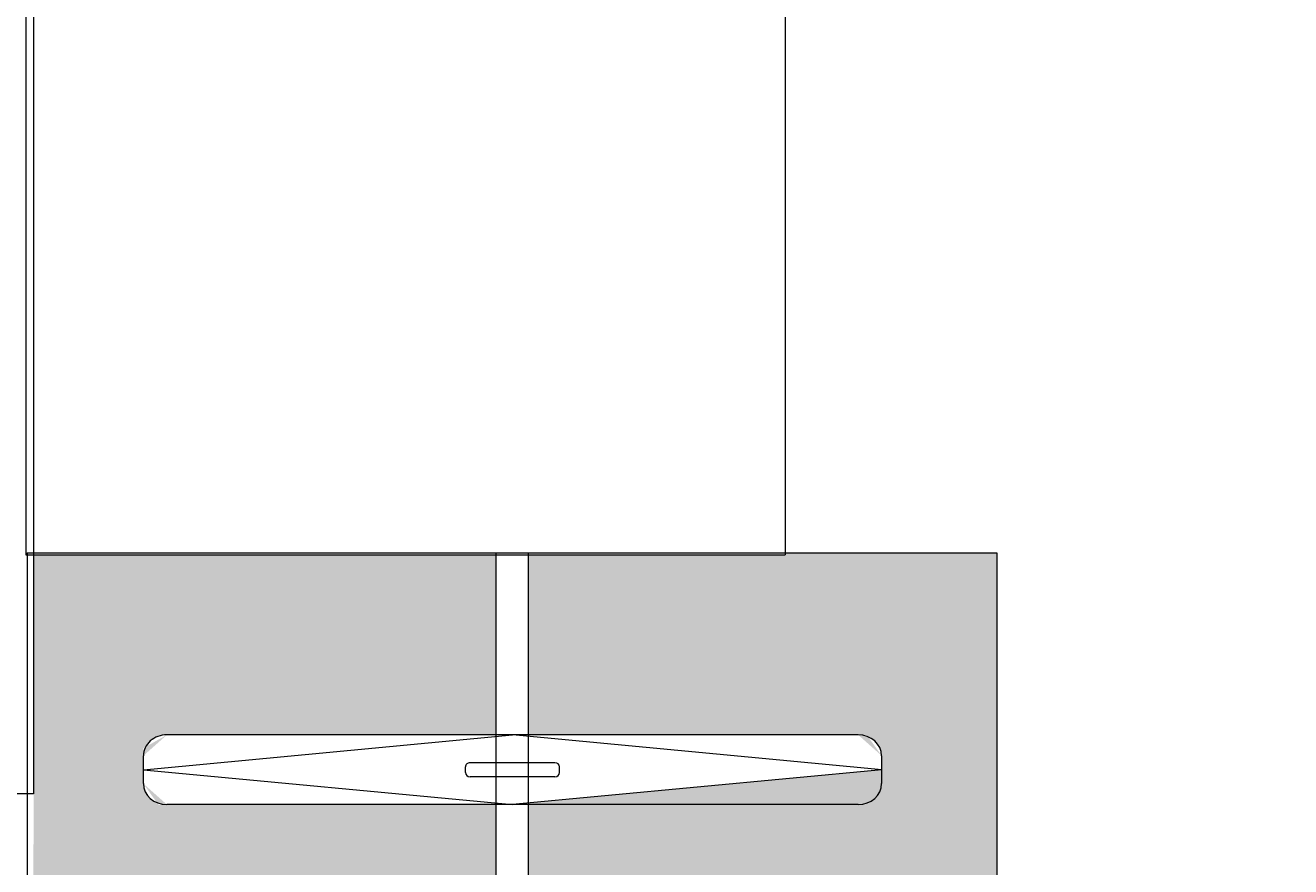
# Model space of a CAD drawing. Units: millimetres. Extents: x 27017497 to 27018854, y 7058029 to 7059154.
# Tile 12 of 91: x 27017623 to 27017651, y 7058200 to 7058219. Entities that reach past the tile are written whole.
import ezdxf

# ---------------------------------------------------------------- set-up
doc = ezdxf.new("R2010")
doc.units = ezdxf.units.MM
for name, color, linetype, lineweight in [('A-ANNO-DIMS', 2, 'Continuous', 18), ('A-FLOR-CASE', 8, 'Continuous', 20), ('A-FLOR-CASE-PATT', 44, 'Continuous', 13), ('A-GLAZ', 4, 'Continuous', 18)]:
    doc.layers.add(name, color=color, linetype=linetype, lineweight=lineweight)
doc.styles.get("Standard").update_dxf_attribs({"font": 'arial.ttf'})
doc.dimstyles.get("Standard").update_dxf_attribs({"dimtxt": 0.18, "dimasz": 0.18, "dimexe": 0.18, "dimexo": 0.0625, "dimgap": 0.09, "dimtad": 0, "dimtih": 1, "dimtoh": 1, "dimdec": 4, "dimzin": 0, "dimdsep": 46, "dimtxsty": 'Standard', "dimcen": 0.09, "dimadec": 0, "dimazin": 0, "dimtfac": 1, "dimtdec": 4, "dimtofl": 0, "dimtmove": 0, "dimatfit": 3, "dimfxl": 1, "dimtolj": 1, "dimtzin": 0, "dimarcsym": 0})

# ---------------------------------------------------------------- blocks, each defined once
blk = doc.blocks.new('WARDROBE-HANGING')
for p, q in [((0, 21.737), (65.212, 21.737)), ((0, 0), (0, 21.737)), ((4.862, 19.153), (4.08, 10.877)), ((5.175, 19.153), (4.549, 19.153)), ((4.862, 19.153), (5.645, 10.877)), ((4.08, 18.624), (4.08, 3.13)), ((5.645, 18.624), (5.645, 3.13)), ((4.925, 11.934), (4.8, 11.934)), ((4.706, 11.828), (4.706, 9.927)), ((5.019, 11.828), (5.019, 9.927)), ((0, 11.231), (65.212, 11.231)), ((4.862, 2.602), (4.08, 10.877)), ((4.862, 2.602), (5.645, 10.877)), ((0, 10.506), (65.212, 10.506)), ((4.925, 9.821), (4.8, 9.821)), ((5.175, 2.602), (4.549, 2.602)), ((0, 0), (65.212, 0))]:
    blk.add_line(p, q)
for centre, major_axis, start_param, end_param in [((4.549, 18.624), (0, 0.528), 0, 1.570796), ((5.175, 18.624), (0, 0.528), 4.712389, 6.283185), ((4.8, 11.828), (0, 0.106), 0, 1.570796), ((4.925, 11.828), (0, 0.106), -1.570796, 0), ((4.8, 9.927), (0, 0.106), 1.570796, 3.141593), ((4.925, 9.927), (0, 0.106), 3.141593, 4.712389), ((4.549, 3.13), (0, 0.528), 1.570796, 3.141593), ((5.175, 3.13), (0, 0.528), 3.141593, 4.712389)]:
    blk.add_ellipse(centre, major_axis=major_axis, ratio=0.888892, start_param=start_param, end_param=end_param)
blk = doc.blocks.new('WINDOW-SINGLE-LIGHT')
blk.add_lwpolyline([(36, 4.5), (36, 0), (0, 0), (0, 9), (36, 9), (36, 4.5), (0, 4.5)])
blk = doc.blocks.new('*D47')
at = {"layer": 'A-ANNO-DIMS', "color": 0, "lineweight": -2, "transparency": 16777216}
for p, q in [((27017561.166, 7058294.35), (27017561.166, 7058028.6)), ((27018790.606, 7058294.35), (27018790.606, 7058028.6)), ((27017561.346, 7058028.78), (27018175.431, 7058028.78)), ((27018790.426, 7058028.78), (27018176.341, 7058028.78))]:
    blk.add_line(p, q, dxfattribs=at)
at = {"layer": 'A-ANNO-DIMS', "color": 0, "transparency": 16777216}
for points in [[(27017561.346, 7058028.81), (27017561.346, 7058028.75), (27017561.166, 7058028.78)], [(27018790.426, 7058028.81), (27018790.426, 7058028.75), (27018790.606, 7058028.78)]]:
    blk.add_solid(points, dxfattribs=at)
at = {"layer": 'Defpoints', "color": 0, "transparency": 16777216}
for p in [(27017561.166, 7058294.412), (27018790.606, 7058294.412), (27018790.606, 7058028.78)]:
    blk.add_point(p, dxfattribs=at)
at = {"layer": 'A-ANNO-DIMS', "color": 0, "transparency": 16777216, "insert": (27018175.886, 7058028.78), "char_height": 0.18, "attachment_point": 5}
blk.add_mtext('\\A1;1229.4', dxfattribs=at)
blk = doc.blocks.new('*D48')
at = {"layer": 'A-ANNO-DIMS', "color": 0, "lineweight": -2, "transparency": 16777216}
for p, q in [((27018463.498, 7058622.912), (27017497.536, 7058622.912)), ((27017497.716, 7058622.732), (27017497.716, 7058357.753)), ((27017497.716, 7058092.41), (27017497.716, 7058357.389)), ((27018555.129, 7058092.23), (27017497.536, 7058092.23))]:
    blk.add_line(p, q, dxfattribs=at)
at = {"layer": 'A-ANNO-DIMS', "color": 0, "transparency": 16777216}
for points in [[(27017497.686, 7058622.732), (27017497.746, 7058622.732), (27017497.716, 7058622.912)], [(27017497.686, 7058092.41), (27017497.746, 7058092.41), (27017497.716, 7058092.23)]]:
    blk.add_solid(points, dxfattribs=at)
at = {"layer": 'Defpoints', "color": 0, "transparency": 16777216}
for p in [(27018463.561, 7058622.912), (27017497.716, 7058092.23), (27018555.192, 7058092.23)]:
    blk.add_point(p, dxfattribs=at)
at = {"layer": 'A-ANNO-DIMS', "color": 0, "transparency": 16777216, "insert": (27017497.716, 7058357.571), "char_height": 0.18, "attachment_point": 5}
blk.add_mtext('\\A1;530.7', dxfattribs=at)

msp = doc.modelspace()

# ---------------------------------------------------------------- hatches: boundary and pattern name
at = {"layer": 'A-FLOR-CASE-PATT'}
h = msp.add_hatch(color=256, dxfattribs=at)
h.dxf.hatch_style = 1
edge = h.paths.add_edge_path()
edge.add_line((27017644.461, 7058207.1), (27017639.716, 7058207.1))
edge.add_line((27017639.716, 7058207.1), (27017639.716, 7058207.055))
edge.add_line((27017639.716, 7058207.055), (27017633.955, 7058207.055))
edge.add_line((27017633.955, 7058207.055), (27017633.955, 7058203.02))
edge.add_line((27017633.955, 7058203.02), (27017641.542, 7058203.02))
edge.add_ellipse((27017641.349, 7058202.551), major_axis=(0.528, 0), ratio=0.888892, start_angle=0, end_angle=90, ccw=False)
edge.add_line((27017641.877, 7058202.551), (27017641.877, 7058202.238))
edge.add_line((27017641.877, 7058202.238), (27017633.955, 7058201.488))
edge.add_line((27017633.955, 7058201.488), (27017633.955, 7058199.747))
edge.add_line((27017633.955, 7058199.747), (27017641.542, 7058199.747))
edge.add_ellipse((27017641.349, 7058199.277), major_axis=(0.528, 0), ratio=0.888892, start_angle=0, end_angle=90, ccw=False)
edge.add_line((27017641.877, 7058199.277), (27017641.877, 7058198.964))
edge.add_line((27017641.877, 7058198.964), (27017633.955, 7058198.215))
edge.add_line((27017633.955, 7058198.215), (27017633.955, 7058193.415))
edge.add_line((27017633.955, 7058193.415), (27017641.403, 7058190.704))
edge.add_ellipse((27017641.06, 7058190.329), major_axis=(0.496, -0.181), ratio=0.888892, start_angle=0, end_angle=90, ccw=False)
edge.add_line((27017641.557, 7058190.148), (27017641.45, 7058189.854))
edge.add_line((27017641.45, 7058189.854), (27017633.955, 7058191.806))
edge.add_line((27017633.955, 7058191.806), (27017633.955, 7058188.22))
edge.add_line((27017633.955, 7058188.22), (27017641.542, 7058188.22))
edge.add_ellipse((27017641.349, 7058187.75), major_axis=(0.528, 0), ratio=0.888892, start_angle=0, end_angle=90, ccw=False)
edge.add_line((27017641.877, 7058187.75), (27017641.877, 7058187.437))
edge.add_line((27017641.877, 7058187.437), (27017633.955, 7058186.688))
edge.add_line((27017633.955, 7058186.688), (27017633.955, 7058181.982))
edge.add_line((27017633.955, 7058181.982), (27017641.542, 7058181.982))
edge.add_ellipse((27017641.349, 7058181.513), major_axis=(0.528, 0), ratio=0.888892, start_angle=0, end_angle=90, ccw=False)
edge.add_line((27017641.877, 7058181.513), (27017641.877, 7058181.199))
edge.add_line((27017641.877, 7058181.199), (27017633.955, 7058180.45))
edge.add_line((27017633.955, 7058180.45), (27017633.955, 7058178.709))
edge.add_line((27017633.955, 7058178.709), (27017641.542, 7058178.709))
edge.add_ellipse((27017641.349, 7058178.239), major_axis=(0.528, 0), ratio=0.888892, start_angle=0, end_angle=90, ccw=False)
edge.add_line((27017641.877, 7058178.239), (27017641.877, 7058177.926))
edge.add_line((27017641.877, 7058177.926), (27017633.955, 7058177.177))
edge.add_line((27017633.955, 7058177.177), (27017633.955, 7058173.878))
edge.add_line((27017633.955, 7058173.878), (27017641.403, 7058171.167))
edge.add_ellipse((27017641.06, 7058170.792), major_axis=(0.496, -0.181), ratio=0.888892, start_angle=0, end_angle=90, ccw=False)
edge.add_line((27017641.557, 7058170.611), (27017641.45, 7058170.317))
edge.add_line((27017641.45, 7058170.317), (27017633.955, 7058172.269))
edge.add_line((27017633.955, 7058172.269), (27017633.955, 7058168.293))
edge.add_line((27017633.955, 7058168.293), (27017641.542, 7058168.293))
edge.add_ellipse((27017641.349, 7058167.824), major_axis=(0.528, 0), ratio=0.888892, start_angle=0, end_angle=90, ccw=False)
edge.add_line((27017641.877, 7058167.824), (27017641.877, 7058167.511))
edge.add_line((27017641.877, 7058167.511), (27017633.955, 7058166.762))
edge.add_line((27017633.955, 7058166.762), (27017633.955, 7058160.389))
edge.add_line((27017633.955, 7058160.389), (27017641.542, 7058160.389))
edge.add_ellipse((27017641.349, 7058159.92), major_axis=(0.528, 0), ratio=0.888892, start_angle=0, end_angle=90, ccw=False)
edge.add_line((27017641.877, 7058159.92), (27017641.877, 7058159.607))
edge.add_line((27017641.877, 7058159.607), (27017633.955, 7058158.858))
edge.add_line((27017633.955, 7058158.858), (27017633.955, 7058157.116))
edge.add_line((27017633.955, 7058157.116), (27017641.542, 7058157.116))
edge.add_ellipse((27017641.349, 7058156.647), major_axis=(0.528, 0), ratio=0.888892, start_angle=0, end_angle=90, ccw=False)
edge.add_line((27017641.877, 7058156.647), (27017641.877, 7058156.334))
edge.add_line((27017641.877, 7058156.334), (27017633.955, 7058155.585))
edge.add_line((27017633.955, 7058155.585), (27017633.955, 7058150.784))
edge.add_line((27017633.955, 7058150.784), (27017641.403, 7058148.073))
edge.add_ellipse((27017641.06, 7058147.698), major_axis=(0.496, -0.181), ratio=0.888892, start_angle=0, end_angle=90, ccw=False)
edge.add_line((27017641.557, 7058147.517), (27017641.45, 7058147.223))
edge.add_line((27017641.45, 7058147.223), (27017633.955, 7058149.175))
edge.add_line((27017633.955, 7058149.175), (27017633.955, 7058145.589))
edge.add_line((27017633.955, 7058145.589), (27017641.542, 7058145.589))
edge.add_ellipse((27017641.349, 7058145.119), major_axis=(0.528, 0), ratio=0.888892, start_angle=0, end_angle=90, ccw=False)
edge.add_line((27017641.877, 7058145.119), (27017641.877, 7058144.806))
edge.add_line((27017641.877, 7058144.806), (27017633.955, 7058144.057))
edge.add_line((27017633.955, 7058144.057), (27017633.955, 7058141.912))
edge.add_line((27017633.955, 7058141.912), (27017644.461, 7058141.912))
edge.add_line((27017644.461, 7058141.912), (27017644.461, 7058207.1))
edge = h.paths.add_edge_path()
edge.add_ellipse((27017626.287, 7058195.04), major_axis=(0.496, -0.181), ratio=0.888892, start_angle=180, end_angle=270, ccw=False)
edge.add_line((27017625.79, 7058195.22), (27017626.063, 7058195.97))
edge.add_ellipse((27017626.501, 7058195.628), major_axis=(0.496, -0.181), ratio=0.888892, start_angle=90, end_angle=180, ccw=False)
edge.add_line((27017626.661, 7058196.069), (27017633.23, 7058193.678))
edge.add_line((27017633.23, 7058193.678), (27017633.23, 7058198.182))
edge.add_line((27017633.23, 7058198.182), (27017625.661, 7058198.182))
edge.add_ellipse((27017625.854, 7058198.651), major_axis=(0.528, 0), ratio=0.888892, start_angle=180, end_angle=270, ccw=False)
edge.add_line((27017625.326, 7058198.651), (27017625.326, 7058199.449))
edge.add_ellipse((27017625.854, 7058199.277), major_axis=(0.528, 0), ratio=0.888892, start_angle=90, end_angle=180, ccw=False)
edge.add_line((27017625.854, 7058199.747), (27017633.23, 7058199.747))
edge.add_line((27017633.23, 7058199.747), (27017633.23, 7058201.455))
edge.add_line((27017633.23, 7058201.455), (27017625.661, 7058201.455))
edge.add_ellipse((27017625.854, 7058201.924), major_axis=(0.528, 0), ratio=0.888892, start_angle=180, end_angle=270, ccw=False)
edge.add_line((27017625.326, 7058201.924), (27017625.326, 7058202.722))
edge.add_ellipse((27017625.854, 7058202.551), major_axis=(0.528, 0), ratio=0.888892, start_angle=90, end_angle=180, ccw=False)
edge.add_line((27017625.854, 7058203.02), (27017633.23, 7058203.02))
edge.add_line((27017633.23, 7058203.02), (27017633.23, 7058207.055))
edge.add_line((27017633.23, 7058207.055), (27017622.865, 7058207.055))
edge.add_line((27017622.865, 7058207.055), (27017622.865, 7058201.7))
edge.add_line((27017622.865, 7058201.7), (27017622.724, 7058141.912))
edge.add_line((27017622.724, 7058141.912), (27017633.23, 7058141.912))
edge.add_line((27017633.23, 7058141.912), (27017633.23, 7058144.024))
edge.add_line((27017633.23, 7058144.024), (27017625.661, 7058144.024))
edge.add_ellipse((27017625.854, 7058144.493), major_axis=(0.528, 0), ratio=0.888892, start_angle=180, end_angle=270, ccw=False)
edge.add_line((27017625.326, 7058144.493), (27017625.326, 7058145.291))
edge.add_ellipse((27017625.854, 7058145.119), major_axis=(0.528, 0), ratio=0.888892, start_angle=90, end_angle=180, ccw=False)
edge.add_line((27017625.854, 7058145.589), (27017633.23, 7058145.589))
edge.add_line((27017633.23, 7058145.589), (27017633.23, 7058149.382))
edge.add_line((27017633.23, 7058149.382), (27017625.944, 7058152.034))
edge.add_ellipse((27017626.287, 7058152.409), major_axis=(0.496, -0.181), ratio=0.888892, start_angle=180, end_angle=270, ccw=False)
edge.add_line((27017625.79, 7058152.59), (27017626.063, 7058153.34))
edge.add_ellipse((27017626.501, 7058152.997), major_axis=(0.496, -0.181), ratio=0.888892, start_angle=90, end_angle=180, ccw=False)
edge.add_line((27017626.661, 7058153.439), (27017633.23, 7058151.048))
edge.add_line((27017633.23, 7058151.048), (27017633.23, 7058155.551))
edge.add_line((27017633.23, 7058155.551), (27017625.661, 7058155.551))
edge.add_ellipse((27017625.854, 7058156.021), major_axis=(0.528, 0), ratio=0.888892, start_angle=180, end_angle=270, ccw=False)
edge.add_line((27017625.326, 7058156.021), (27017625.326, 7058156.819))
edge.add_ellipse((27017625.854, 7058156.647), major_axis=(0.528, 0), ratio=0.888892, start_angle=90, end_angle=180, ccw=False)
edge.add_line((27017625.854, 7058157.116), (27017633.23, 7058157.116))
edge.add_line((27017633.23, 7058157.116), (27017633.23, 7058158.824))
edge.add_line((27017633.23, 7058158.824), (27017625.661, 7058158.824))
edge.add_ellipse((27017625.854, 7058159.294), major_axis=(0.528, 0), ratio=0.888892, start_angle=180, end_angle=270, ccw=False)
edge.add_line((27017625.326, 7058159.294), (27017625.326, 7058160.092))
edge.add_ellipse((27017625.854, 7058159.92), major_axis=(0.528, 0), ratio=0.888892, start_angle=90, end_angle=180, ccw=False)
edge.add_line((27017625.854, 7058160.389), (27017633.23, 7058160.389))
edge.add_line((27017633.23, 7058160.389), (27017633.23, 7058166.728))
edge.add_line((27017633.23, 7058166.728), (27017625.661, 7058166.728))
edge.add_ellipse((27017625.854, 7058167.198), major_axis=(0.528, 0), ratio=0.888892, start_angle=180, end_angle=270, ccw=False)
edge.add_line((27017625.326, 7058167.198), (27017625.326, 7058167.996))
edge.add_ellipse((27017625.854, 7058167.824), major_axis=(0.528, 0), ratio=0.888892, start_angle=90, end_angle=180, ccw=False)
edge.add_line((27017625.854, 7058168.293), (27017633.23, 7058168.293))
edge.add_line((27017633.23, 7058168.293), (27017633.23, 7058172.476))
edge.add_line((27017633.23, 7058172.476), (27017625.944, 7058175.128))
edge.add_ellipse((27017626.287, 7058175.503), major_axis=(0.496, -0.181), ratio=0.888892, start_angle=180, end_angle=270, ccw=False)
edge.add_line((27017625.79, 7058175.684), (27017626.063, 7058176.433))
edge.add_ellipse((27017626.501, 7058176.091), major_axis=(0.496, -0.181), ratio=0.888892, start_angle=90, end_angle=180, ccw=False)
edge.add_line((27017626.661, 7058176.533), (27017633.23, 7058174.142))
edge.add_line((27017633.23, 7058174.142), (27017633.23, 7058177.144))
edge.add_line((27017633.23, 7058177.144), (27017625.661, 7058177.144))
edge.add_ellipse((27017625.854, 7058177.613), major_axis=(0.528, 0), ratio=0.888892, start_angle=180, end_angle=270, ccw=False)
edge.add_line((27017625.326, 7058177.613), (27017625.326, 7058178.411))
edge.add_ellipse((27017625.854, 7058178.239), major_axis=(0.528, 0), ratio=0.888892, start_angle=90, end_angle=180, ccw=False)
edge.add_line((27017625.854, 7058178.709), (27017633.23, 7058178.709))
edge.add_line((27017633.23, 7058178.709), (27017633.23, 7058180.417))
edge.add_line((27017633.23, 7058180.417), (27017625.661, 7058180.417))
edge.add_ellipse((27017625.854, 7058180.886), major_axis=(0.528, 0), ratio=0.888892, start_angle=180, end_angle=270, ccw=False)
edge.add_line((27017625.326, 7058180.886), (27017625.326, 7058181.684))
edge.add_ellipse((27017625.854, 7058181.513), major_axis=(0.528, 0), ratio=0.888892, start_angle=90, end_angle=180, ccw=False)
edge.add_line((27017625.854, 7058181.982), (27017633.23, 7058181.982))
edge.add_line((27017633.23, 7058181.982), (27017633.23, 7058186.655))
edge.add_line((27017633.23, 7058186.655), (27017625.661, 7058186.655))
edge.add_ellipse((27017625.854, 7058187.124), major_axis=(0.528, 0), ratio=0.888892, start_angle=180, end_angle=270, ccw=False)
edge.add_line((27017625.326, 7058187.124), (27017625.326, 7058187.922))
edge.add_ellipse((27017625.854, 7058187.75), major_axis=(0.528, 0), ratio=0.888892, start_angle=90, end_angle=180, ccw=False)
edge.add_line((27017625.854, 7058188.22), (27017633.23, 7058188.22))
edge.add_line((27017633.23, 7058188.22), (27017633.23, 7058192.013))
edge.add_line((27017633.23, 7058192.013), (27017625.944, 7058194.665))

# ---------------------------------------------------------------- linework, layer by layer
at = {"layer": 'A-FLOR-CASE'}
for p, q in [((27017639.716, 7058294.412), (27017639.716, 7058207.055)), ((27017622.691, 7058258.237), (27017622.691, 7058207.055)), ((27017622.691, 7058207.055), (27017639.716, 7058207.055))]:
    msp.add_line(p, q, dxfattribs=at)

# ---------------------------------------------------------------- block references
at = {"layer": 'A-FLOR-CASE', "rotation": 270}
msp.add_blockref('WARDROBE-HANGING', (27017622.724, 7058207.1), dxfattribs=at)
at = {"layer": 'A-GLAZ', "rotation": 270}
msp.add_blockref('WINDOW-SINGLE-LIGHT', (27017613.865, 7058237.7), dxfattribs=at)

# ---------------------------------------------------------------- dimensions: what is measured, and where the dimension line sits
at = {"layer": 'A-ANNO-DIMS'}
dim = msp.add_linear_dim(base=(27017497.716, 7058092.23), p1=(27018463.561, 7058622.912), p2=(27018555.192, 7058092.23), angle=90, dimstyle='Standard', override={"dimdec": 1, "dimlfac": 1, "dimrnd": 0, "dimzin": 0, "dimdsep": 46, "dimlunit": 2}, dxfattribs=at)
dim.commit()
dim.dimension.update_dxf_attribs({"geometry": '*D48', "text_midpoint": (27017497.716, 7058357.571)})
dim = msp.add_linear_dim(base=(27018790.606, 7058028.78), p1=(27017561.166, 7058294.412), p2=(27018790.606, 7058294.412), dimstyle='Standard', override={"dimdec": 1, "dimlfac": 1, "dimrnd": 0, "dimzin": 0, "dimdsep": 46, "dimlunit": 2}, dxfattribs=at)
dim.commit()
dim.dimension.update_dxf_attribs({"geometry": '*D47', "text_midpoint": (27018175.886, 7058028.78)})

doc.saveas('drawing.dxf')
